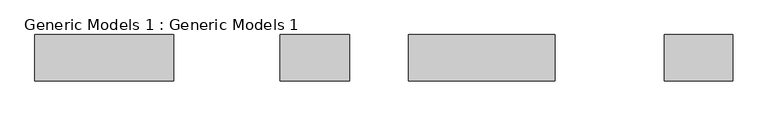
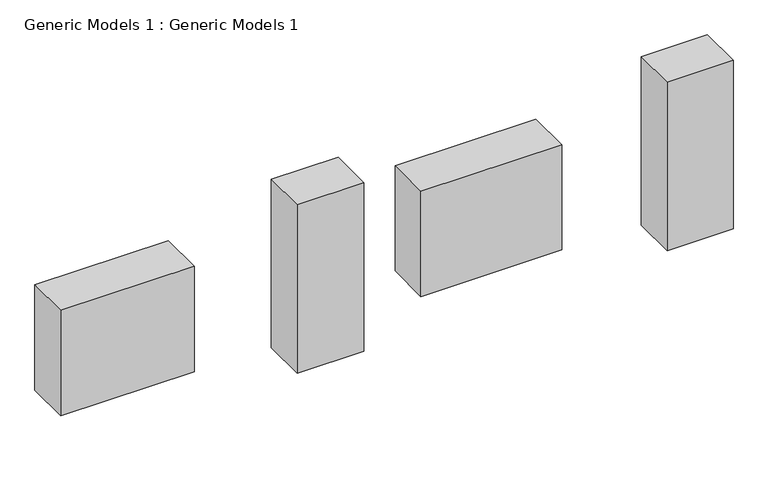
"""IFC4 building model written with IfcOpenShell, lengths in millimetres: proxy geometry, Generic Models 1 : Generic Models 1."""

from ifc_helpers import new_model, si_unit, frame, origin, place, context, project, spatial, polyline, outline, extrude, source, transform, mapped, element, save


def generic_models_1_generic_models_1_f3bdfb45(model_context):
    return source(origin(), model_context, "Body", "SweptSolid", [
        extrude(outline(polyline([(-5924.0910991, -10043.743996), (-6838.4910991, -10043.743996), (-6838.4910991, -9738.943996), (-5924.0910991, -9738.943996), (-5924.0910991, -10043.743996)])), frame((0.0, 0.0, 380.9257259), z_axis=(0.0, 0.0, 1.0), x_axis=(1.0, 0.0, 0.0)), (0.0, 0.0, 1.0), 762.0),
        extrude(outline(polyline([(-4762.8939058, -10043.743996), (-5220.0939058, -10043.743996), (-5220.0939058, -9738.943996), (-4762.8939058, -9738.943996), (-4762.8939058, -10043.743996)])), frame((0.0, 0.0, 121.6930433), z_axis=(0.0, 0.0, 1.0), x_axis=(1.0, 0.0, 0.0)), (0.0, 0.0, 1.0), 1219.2),
        extrude(outline(polyline([(-3408.8307258, -10043.743996), (-4373.1606596, -10043.743996), (-4373.1606596, -9738.943996), (-3408.8307258, -9738.943996), (-3408.8307258, -10043.743996)])), frame((0.0, 0.0, 380.9257259), z_axis=(0.0, 0.0, 1.0), x_axis=(1.0, 0.0, 0.0)), (0.0, 0.0, 1.0), 762.0),
        extrude(outline(polyline([(-2235.1050693, -10043.743996), (-2687.2192603, -10043.743996), (-2687.2192603, -9738.943996), (-2235.1050693, -9738.943996), (-2235.1050693, -10043.743996)])), frame((0.0, 0.0, 121.6930433), z_axis=(0.0, 0.0, 1.0), x_axis=(1.0, 0.0, 0.0)), (0.0, 0.0, 1.0), 1219.2),
    ])


if __name__ == "__main__":
    model = new_model("IFC4")
    model_context = context("Model", 3, world=origin())
    ifc_project = project(units=[si_unit("LENGTHUNIT", "METRE", prefix="MILLI")], contexts=[model_context])
    site = spatial("IfcSite", under=ifc_project)
    building = spatial("IfcBuilding", under=site)
    placement = place(None, origin())
    generic_models_1_generic_models_1_shape = generic_models_1_generic_models_1_f3bdfb45(model_context)
    element("IfcBuildingElementProxy", 1, Name="Generic Models 1 : Generic Models 1", ObjectType="Generic Models 1 : Generic Models 1", at=placement, inside=building, context=model_context, shape_type="MappedRepresentation", body=[
        mapped(generic_models_1_generic_models_1_shape, transform((0.0, 0.0, 0.0), x_axis=(1.0, 0.0, 0.0), y_axis=(0.0, 1.0, 0.0), z_axis=(0.0, 0.0, 1.0))),
    ])
    save(model, "model.ifc")

# Revit data of these elements
# Element 1 (IfcBuildingElementProxy, "Generic Models 1 : Generic Models 1")
#   Materials on its faces: "Brick, Common"
# Materials
#   "Brick, Common": class "Masonry", colour RGB 170 98 104, transparency 0, Description = "Common brick", Cost = 0
